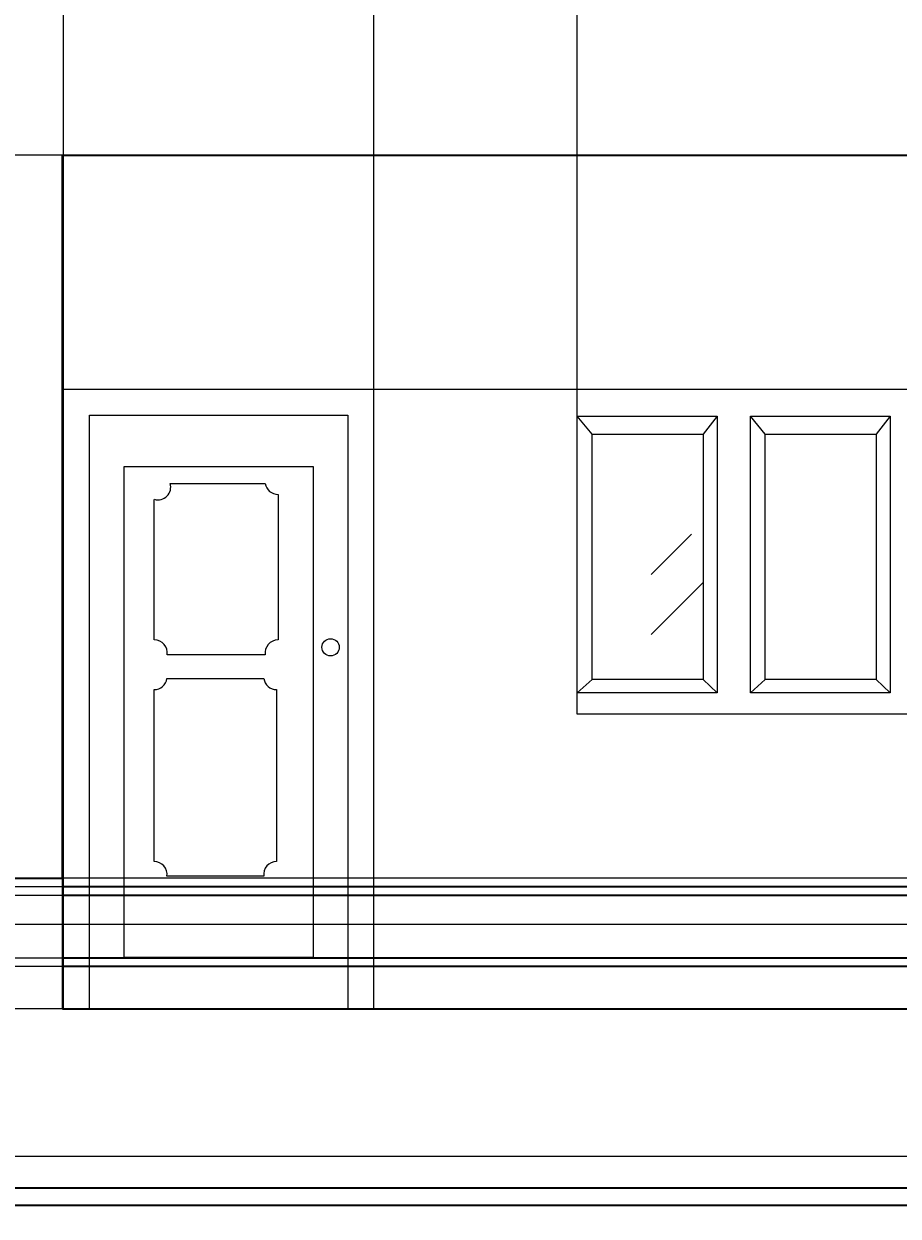
# Model space of a CAD drawing. Units: inches. Extents: x 93 to 565, y 123 to 656.
# Tile 9 of 18: x 291 to 393, y 324 to 463. Entities that reach past the tile are written whole.
import ezdxf

# ---------------------------------------------------------------- set-up
doc = ezdxf.new("R2010")
doc.units = ezdxf.units.IN
doc.header["$MEASUREMENT"] = 0
for name, color, linetype, lineweight in [('A-ANNO-DIMS', 2, 'Continuous', 18), ('A-DOOR', 3, 'Continuous', 25), ('A-ELEV', 7, 'Continuous', 35), ('A-GLAZ', 4, 'Continuous', 25)]:
    doc.layers.add(name, color=color, linetype=linetype, lineweight=lineweight)
doc.styles.get("Standard").update_dxf_attribs({"font": 'arial.ttf'})
doc.dimstyles.get("Standard").update_dxf_attribs({"dimtxt": 0.18, "dimasz": 0.18, "dimexe": 0.18, "dimexo": 0.0625, "dimgap": 0.09, "dimtad": 0, "dimtih": 1, "dimtoh": 1, "dimdec": 4, "dimzin": 0, "dimdsep": 46, "dimtxsty": 'Standard', "dimcen": 0.09, "dimadec": 0, "dimazin": 0, "dimtfac": 1, "dimtdec": 4, "dimtofl": 0, "dimtmove": 0, "dimatfit": 3, "dimfxl": 1, "dimtolj": 1, "dimtzin": 0, "dimarcsym": 0})

# ---------------------------------------------------------------- blocks, each defined once
blk = doc.blocks.new('*U10')
blk.add_lwpolyline([(3.12, 0.01), (0.12, 0.01), (0.12, 72.01), (36.12, 72.01), (36.12, 0.01), (33.12, 0.01)])
for points in [[(33.12, 68.99), (33.12, 0.01), (3.12, 0.01), (3.12, 68.99)], [(29.12, 6.01), (29.12, 62.99), (7.12, 62.99), (7.12, 6.01)]]:
    blk.add_lwpolyline(points, close=True)
blk.add_circle((31.12, 42.01), 1)
blk = doc.blocks.new('DOOR-PANEL-UPPER')
for points in [[(1.85, 19.9), (12.89, 19.9)], [(0, 1.72), (0, 18.05)], [(14.37, 18.62), (14.37, 1.72)], [(12.89, 0), (1.48, 0)]]:
    blk.add_lwpolyline(points)
for centre, start, end in [((0.41, 19.5), 254.1895, 15.8285), ((14.37, 20.12), 188.4141, 270), ((0, 0.22), 351.5859, 90), ((14.37, 0.22), 90, 188.4141)]:
    blk.add_arc(centre, 1.5, start, end)
blk = doc.blocks.new('DOOR-PANEL-LOWER')
for points in [[(1.48, 22.97), (12.73, 22.97)], [(0, 1.72), (0, 21.69)], [(14.21, 21.69), (14.21, 1.72)], [(12.73, 0), (1.48, 0)]]:
    blk.add_lwpolyline(points)
for centre, start, end in [((0, 23.19), 270, 351.5859), ((14.21, 23.19), 188.4141, 270), ((0, 0.22), 351.5859, 90), ((14.21, 0.22), 90, 188.4141)]:
    blk.add_arc(centre, 1.5, start, end)
blk = doc.blocks.new('WIN-CASEMENT-SMALL')
blk.add_lwpolyline([(1.71, 28.48), (0, 30.59), (16.23, 30.59), (14.61, 28.48)])
blk.add_lwpolyline([(1.71, 28.48), (14.61, 28.48), (14.61, 0), (1.71, 0)], close=True)
blk = doc.blocks.new('*D28')
at = {"layer": 'A-ANNO-DIMS', "color": 0, "lineweight": -2, "transparency": 16777216}
for p, q in [((210.54, 519.04), (210.54, 134)), ((295.69, 183.67), (295.69, 134)), ((210.72, 134.18), (252.72, 134.18)), ((295.51, 134.18), (253.51, 134.18))]:
    blk.add_line(p, q, dxfattribs=at)
at = {"layer": 'A-ANNO-DIMS', "color": 0, "transparency": 16777216}
for points in [[(210.72, 134.21), (210.72, 134.15), (210.54, 134.18)], [(295.51, 134.21), (295.51, 134.15), (295.69, 134.18)]]:
    blk.add_solid(points, dxfattribs=at)
at = {"layer": 'Defpoints', "color": 0, "transparency": 16777216}
for p in [(210.54, 519.1), (295.69, 183.73), (295.69, 134.18)]:
    blk.add_point(p, dxfattribs=at)
at = {"layer": 'A-ANNO-DIMS', "color": 0, "transparency": 16777216, "insert": (253.12, 134.18), "char_height": 0.18, "attachment_point": 5}
blk.add_mtext('\\A1;85.14', dxfattribs=at)
blk = doc.blocks.new('*D29')
at = {"layer": 'A-ANNO-DIMS', "color": 0, "lineweight": -2, "transparency": 16777216}
for p, q in [((437.19, 594.34), (437.19, 134)), ((295.69, 183.67), (295.69, 134)), ((295.87, 134.18), (366.05, 134.18)), ((437.01, 134.18), (366.82, 134.18))]:
    blk.add_line(p, q, dxfattribs=at)
at = {"layer": 'A-ANNO-DIMS', "color": 0, "transparency": 16777216}
for points in [[(295.87, 134.21), (295.87, 134.15), (295.69, 134.18)], [(437.01, 134.21), (437.01, 134.15), (437.19, 134.18)]]:
    blk.add_solid(points, dxfattribs=at)
at = {"layer": 'Defpoints', "color": 0, "transparency": 16777216}
for p in [(437.19, 594.4), (295.69, 183.73), (437.19, 134.18)]:
    blk.add_point(p, dxfattribs=at)
at = {"layer": 'A-ANNO-DIMS', "color": 0, "transparency": 16777216, "insert": (366.44, 134.18), "char_height": 0.18, "attachment_point": 5}
blk.add_mtext('\\A1;141.5', dxfattribs=at)
blk = doc.blocks.new('*D31')
at = {"layer": 'A-ANNO-DIMS', "color": 0, "lineweight": -2, "transparency": 16777216}
for p, q in [((417.87, 630.4), (564.81, 630.4)), ((564.63, 630.22), (564.63, 395.25)), ((564.63, 159.91), (564.63, 394.89)), ((119.14, 159.73), (564.81, 159.73))]:
    blk.add_line(p, q, dxfattribs=at)
at = {"layer": 'A-ANNO-DIMS', "color": 0, "transparency": 16777216}
for points in [[(564.6, 630.22), (564.66, 630.22), (564.63, 630.4)], [(564.6, 159.91), (564.66, 159.91), (564.63, 159.73)]]:
    blk.add_solid(points, dxfattribs=at)
at = {"layer": 'Defpoints', "color": 0, "transparency": 16777216}
for p in [(417.81, 630.4), (564.63, 630.4), (119.08, 159.73)]:
    blk.add_point(p, dxfattribs=at)
at = {"layer": 'A-ANNO-DIMS', "color": 0, "transparency": 16777216, "insert": (564.63, 395.07), "char_height": 0.18, "attachment_point": 5}
blk.add_mtext('\\A1;470.7', dxfattribs=at)
blk = doc.blocks.new('*D66')
at = {"layer": 'A-ANNO-DIMS', "color": 0, "lineweight": -2, "transparency": 16777216}
for p, q in [((295.81, 420.63), (295.81, 656.13)), ((295.99, 655.95), (313.59, 655.95)), ((331.63, 655.95), (314.03, 655.95)), ((331.81, 420.63), (331.81, 656.13))]:
    blk.add_line(p, q, dxfattribs=at)
at = {"layer": 'A-ANNO-DIMS', "color": 0, "transparency": 16777216}
for points in [[(295.99, 655.98), (295.99, 655.92), (295.81, 655.95)], [(331.63, 655.98), (331.63, 655.92), (331.81, 655.95)]]:
    blk.add_solid(points, dxfattribs=at)
at = {"layer": 'Defpoints', "color": 0, "transparency": 16777216}
for p in [(331.81, 655.95), (295.81, 420.57), (331.81, 420.57)]:
    blk.add_point(p, dxfattribs=at)
at = {"layer": 'A-ANNO-DIMS', "color": 0, "transparency": 16777216, "insert": (313.81, 655.95), "char_height": 0.18, "attachment_point": 5}
blk.add_mtext('\\A1;36', dxfattribs=at)
blk = doc.blocks.new('*D67')
at = {"layer": 'A-ANNO-DIMS', "color": 0, "lineweight": -2, "transparency": 16777216}
for p, q in [((331.87, 420.57), (564.81, 420.57)), ((564.63, 420.39), (564.63, 384.75)), ((564.63, 348.75), (564.63, 384.39)), ((331.87, 348.57), (564.81, 348.57))]:
    blk.add_line(p, q, dxfattribs=at)
at = {"layer": 'A-ANNO-DIMS', "color": 0, "transparency": 16777216}
for points in [[(564.6, 420.39), (564.66, 420.39), (564.63, 420.57)], [(564.6, 348.75), (564.66, 348.75), (564.63, 348.57)]]:
    blk.add_solid(points, dxfattribs=at)
at = {"layer": 'Defpoints', "color": 0, "transparency": 16777216}
for p in [(331.81, 420.57), (564.63, 420.57), (331.81, 348.57)]:
    blk.add_point(p, dxfattribs=at)
at = {"layer": 'A-ANNO-DIMS', "color": 0, "transparency": 16777216, "insert": (564.63, 384.57), "char_height": 0.18, "attachment_point": 5}
blk.add_mtext('\\A1;72', dxfattribs=at)
blk = doc.blocks.new('*D68')
at = {"layer": 'A-ANNO-DIMS', "color": 0, "lineweight": -2, "transparency": 16777216}
for p, q in [((331.81, 420.63), (331.81, 656.13)), ((331.99, 655.95), (343.24, 655.95)), ((355.28, 655.95), (344.03, 655.95)), ((355.46, 420.63), (355.46, 656.13))]:
    blk.add_line(p, q, dxfattribs=at)
at = {"layer": 'A-ANNO-DIMS', "color": 0, "transparency": 16777216}
for points in [[(331.99, 655.98), (331.99, 655.92), (331.81, 655.95)], [(355.28, 655.98), (355.28, 655.92), (355.46, 655.95)]]:
    blk.add_solid(points, dxfattribs=at)
at = {"layer": 'Defpoints', "color": 0, "transparency": 16777216}
for p in [(355.46, 655.95), (331.81, 420.57), (355.46, 420.57)]:
    blk.add_point(p, dxfattribs=at)
at = {"layer": 'A-ANNO-DIMS', "color": 0, "transparency": 16777216, "insert": (343.64, 655.95), "char_height": 0.18, "attachment_point": 5}
blk.add_mtext('\\A1;23.65', dxfattribs=at)
blk = doc.blocks.new('*D69')
at = {"layer": 'A-ANNO-DIMS', "color": 0, "lineweight": -2, "transparency": 16777216}
for p, q in [((355.46, 420.63), (355.46, 656.13)), ((355.64, 655.95), (391.65, 655.95)), ((428.44, 655.95), (392.43, 655.95)), ((428.62, 420.63), (428.62, 656.13))]:
    blk.add_line(p, q, dxfattribs=at)
at = {"layer": 'A-ANNO-DIMS', "color": 0, "transparency": 16777216}
for points in [[(355.64, 655.98), (355.64, 655.92), (355.46, 655.95)], [(428.44, 655.98), (428.44, 655.92), (428.62, 655.95)]]:
    blk.add_solid(points, dxfattribs=at)
at = {"layer": 'Defpoints', "color": 0, "transparency": 16777216}
for p in [(428.62, 655.95), (355.46, 420.57), (428.62, 420.57)]:
    blk.add_point(p, dxfattribs=at)
at = {"layer": 'A-ANNO-DIMS', "color": 0, "transparency": 16777216, "insert": (392.04, 655.95), "char_height": 0.18, "attachment_point": 5}
blk.add_mtext('\\A1;73.16', dxfattribs=at)
blk = doc.blocks.new('*D72')
at = {"layer": 'A-ANNO-DIMS', "color": 0, "lineweight": -2, "transparency": 16777216}
for p, q in [((295.62, 447.73), (93.35, 447.73)), ((93.53, 447.55), (93.53, 405.91)), ((93.53, 363.91), (93.53, 405.55)), ((286.62, 363.73), (93.35, 363.73))]:
    blk.add_line(p, q, dxfattribs=at)
at = {"layer": 'A-ANNO-DIMS', "color": 0, "transparency": 16777216}
for points in [[(93.5, 447.55), (93.56, 447.55), (93.53, 447.73)], [(93.5, 363.91), (93.56, 363.91), (93.53, 363.73)]]:
    blk.add_solid(points, dxfattribs=at)
at = {"layer": 'Defpoints', "color": 0, "transparency": 16777216}
for p in [(295.69, 447.73), (93.53, 363.73), (286.69, 363.73)]:
    blk.add_point(p, dxfattribs=at)
at = {"layer": 'A-ANNO-DIMS', "color": 0, "transparency": 16777216, "insert": (93.53, 405.73), "char_height": 0.18, "attachment_point": 5}
blk.add_mtext('\\A1;84', dxfattribs=at)
blk = doc.blocks.new('*D107')
at = {"layer": 'A-ANNO-DIMS', "color": 0, "lineweight": -2, "transparency": 16777216}
for p, q in [((210.54, 519.04), (210.54, 134)), ((295.69, 183.67), (295.69, 134)), ((210.72, 134.18), (252.65, 134.18)), ((295.51, 134.18), (253.58, 134.18))]:
    blk.add_line(p, q, dxfattribs=at)
at = {"layer": 'A-ANNO-DIMS', "color": 0, "transparency": 16777216}
for points in [[(210.72, 134.21), (210.72, 134.15), (210.54, 134.18)], [(295.51, 134.21), (295.51, 134.15), (295.69, 134.18)]]:
    blk.add_solid(points, dxfattribs=at)
at = {"layer": 'Defpoints', "color": 0, "transparency": 16777216}
for p in [(210.54, 519.1), (295.69, 183.73), (295.69, 134.18)]:
    blk.add_point(p, dxfattribs=at)
at = {"layer": 'A-ANNO-DIMS', "color": 0, "transparency": 16777216, "insert": (253.12, 134.18), "char_height": 0.18, "attachment_point": 5}
blk.add_mtext('\\A1;85.143', dxfattribs=at)
blk = doc.blocks.new('*D108')
at = {"layer": 'A-ANNO-DIMS', "color": 0, "lineweight": -2, "transparency": 16777216}
for p, q in [((437.19, 594.34), (437.19, 134)), ((295.69, 183.67), (295.69, 134)), ((295.87, 134.18), (365.93, 134.18)), ((437.01, 134.18), (366.95, 134.18))]:
    blk.add_line(p, q, dxfattribs=at)
at = {"layer": 'A-ANNO-DIMS', "color": 0, "transparency": 16777216}
for points in [[(295.87, 134.21), (295.87, 134.15), (295.69, 134.18)], [(437.01, 134.21), (437.01, 134.15), (437.19, 134.18)]]:
    blk.add_solid(points, dxfattribs=at)
at = {"layer": 'Defpoints', "color": 0, "transparency": 16777216}
for p in [(437.19, 594.4), (295.69, 183.73), (437.19, 134.18)]:
    blk.add_point(p, dxfattribs=at)
at = {"layer": 'A-ANNO-DIMS', "color": 0, "transparency": 16777216, "insert": (366.44, 134.18), "char_height": 0.18, "attachment_point": 5}
blk.add_mtext('\\A1;141.501', dxfattribs=at)
blk = doc.blocks.new('*D110')
at = {"layer": 'A-ANNO-DIMS', "color": 0, "lineweight": -2, "transparency": 16777216}
for p, q in [((417.87, 630.4), (564.81, 630.4)), ((564.63, 630.22), (564.63, 395.25)), ((564.63, 159.91), (564.63, 394.89)), ((119.14, 159.73), (564.81, 159.73))]:
    blk.add_line(p, q, dxfattribs=at)
at = {"layer": 'A-ANNO-DIMS', "color": 0, "transparency": 16777216}
for points in [[(564.6, 630.22), (564.66, 630.22), (564.63, 630.4)], [(564.6, 159.91), (564.66, 159.91), (564.63, 159.73)]]:
    blk.add_solid(points, dxfattribs=at)
at = {"layer": 'Defpoints', "color": 0, "transparency": 16777216}
for p in [(417.81, 630.4), (564.63, 630.4), (119.08, 159.73)]:
    blk.add_point(p, dxfattribs=at)
at = {"layer": 'A-ANNO-DIMS', "color": 0, "transparency": 16777216, "insert": (564.63, 395.07), "char_height": 0.18, "attachment_point": 5}
blk.add_mtext('\\A1;470.673', dxfattribs=at)
blk = doc.blocks.new('*D145')
at = {"layer": 'A-ANNO-DIMS', "color": 0, "lineweight": -2, "transparency": 16777216}
for p, q in [((295.81, 420.63), (295.81, 656.13)), ((295.99, 655.95), (313.35, 655.95)), ((331.63, 655.95), (314.27, 655.95)), ((331.81, 420.63), (331.81, 656.13))]:
    blk.add_line(p, q, dxfattribs=at)
at = {"layer": 'A-ANNO-DIMS', "color": 0, "transparency": 16777216}
for points in [[(295.99, 655.98), (295.99, 655.92), (295.81, 655.95)], [(331.63, 655.98), (331.63, 655.92), (331.81, 655.95)]]:
    blk.add_solid(points, dxfattribs=at)
at = {"layer": 'Defpoints', "color": 0, "transparency": 16777216}
for p in [(331.81, 655.95), (295.81, 420.57), (331.81, 420.57)]:
    blk.add_point(p, dxfattribs=at)
at = {"layer": 'A-ANNO-DIMS', "color": 0, "transparency": 16777216, "insert": (313.81, 655.95), "char_height": 0.18, "attachment_point": 5}
blk.add_mtext('\\A1;36.000', dxfattribs=at)
blk = doc.blocks.new('*D146')
at = {"layer": 'A-ANNO-DIMS', "color": 0, "lineweight": -2, "transparency": 16777216}
for p, q in [((331.87, 420.57), (564.81, 420.57)), ((564.63, 420.39), (564.63, 384.75)), ((564.63, 348.75), (564.63, 384.39)), ((331.87, 348.57), (564.81, 348.57))]:
    blk.add_line(p, q, dxfattribs=at)
at = {"layer": 'A-ANNO-DIMS', "color": 0, "transparency": 16777216}
for points in [[(564.6, 420.39), (564.66, 420.39), (564.63, 420.57)], [(564.6, 348.75), (564.66, 348.75), (564.63, 348.57)]]:
    blk.add_solid(points, dxfattribs=at)
at = {"layer": 'Defpoints', "color": 0, "transparency": 16777216}
for p in [(331.81, 420.57), (564.63, 420.57), (331.81, 348.57)]:
    blk.add_point(p, dxfattribs=at)
at = {"layer": 'A-ANNO-DIMS', "color": 0, "transparency": 16777216, "insert": (564.63, 384.57), "char_height": 0.18, "attachment_point": 5}
blk.add_mtext('\\A1;72.000', dxfattribs=at)
blk = doc.blocks.new('*D147')
at = {"layer": 'A-ANNO-DIMS', "color": 0, "lineweight": -2, "transparency": 16777216}
for p, q in [((331.81, 420.63), (331.81, 656.13)), ((331.99, 655.95), (343.17, 655.95)), ((355.28, 655.95), (344.1, 655.95)), ((355.46, 420.63), (355.46, 656.13))]:
    blk.add_line(p, q, dxfattribs=at)
at = {"layer": 'A-ANNO-DIMS', "color": 0, "transparency": 16777216}
for points in [[(331.99, 655.98), (331.99, 655.92), (331.81, 655.95)], [(355.28, 655.98), (355.28, 655.92), (355.46, 655.95)]]:
    blk.add_solid(points, dxfattribs=at)
at = {"layer": 'Defpoints', "color": 0, "transparency": 16777216}
for p in [(355.46, 655.95), (331.81, 420.57), (355.46, 420.57)]:
    blk.add_point(p, dxfattribs=at)
at = {"layer": 'A-ANNO-DIMS', "color": 0, "transparency": 16777216, "insert": (343.64, 655.95), "char_height": 0.18, "attachment_point": 5}
blk.add_mtext('\\A1;23.649', dxfattribs=at)
blk = doc.blocks.new('*D148')
at = {"layer": 'A-ANNO-DIMS', "color": 0, "lineweight": -2, "transparency": 16777216}
for p, q in [((355.46, 420.63), (355.46, 656.13)), ((355.64, 655.95), (391.58, 655.95)), ((428.44, 655.95), (392.5, 655.95)), ((428.62, 420.63), (428.62, 656.13))]:
    blk.add_line(p, q, dxfattribs=at)
at = {"layer": 'A-ANNO-DIMS', "color": 0, "transparency": 16777216}
for points in [[(355.64, 655.98), (355.64, 655.92), (355.46, 655.95)], [(428.44, 655.98), (428.44, 655.92), (428.62, 655.95)]]:
    blk.add_solid(points, dxfattribs=at)
at = {"layer": 'Defpoints', "color": 0, "transparency": 16777216}
for p in [(428.62, 655.95), (355.46, 420.57), (428.62, 420.57)]:
    blk.add_point(p, dxfattribs=at)
at = {"layer": 'A-ANNO-DIMS', "color": 0, "transparency": 16777216, "insert": (392.04, 655.95), "char_height": 0.18, "attachment_point": 5}
blk.add_mtext('\\A1;73.156', dxfattribs=at)
blk = doc.blocks.new('*D151')
at = {"layer": 'A-ANNO-DIMS', "color": 0, "lineweight": -2, "transparency": 16777216}
for p, q in [((295.62, 447.73), (93.35, 447.73)), ((93.53, 447.55), (93.53, 405.91)), ((93.53, 363.91), (93.53, 405.55)), ((286.62, 363.73), (93.35, 363.73))]:
    blk.add_line(p, q, dxfattribs=at)
at = {"layer": 'A-ANNO-DIMS', "color": 0, "transparency": 16777216}
for points in [[(93.5, 447.55), (93.56, 447.55), (93.53, 447.73)], [(93.5, 363.91), (93.56, 363.91), (93.53, 363.73)]]:
    blk.add_solid(points, dxfattribs=at)
at = {"layer": 'Defpoints', "color": 0, "transparency": 16777216}
for p in [(295.69, 447.73), (93.53, 363.73), (286.69, 363.73)]:
    blk.add_point(p, dxfattribs=at)
at = {"layer": 'A-ANNO-DIMS', "color": 0, "transparency": 16777216, "insert": (93.53, 405.73), "char_height": 0.18, "attachment_point": 5}
blk.add_mtext('\\A1;84.000', dxfattribs=at)
blk = doc.blocks.new('*D190')
at = {"layer": 'A-ANNO-DIMS', "color": 0, "lineweight": -2, "transparency": 16777216}
for p, q in [((514.58, 348.55), (93.35, 348.55)), ((93.53, 348.37), (93.53, 338.33)), ((93.53, 327.91), (93.53, 337.96)), ((539.02, 327.73), (93.35, 327.73))]:
    blk.add_line(p, q, dxfattribs=at)
at = {"layer": 'A-ANNO-DIMS', "color": 0, "transparency": 16777216}
for points in [[(93.5, 348.37), (93.56, 348.37), (93.53, 348.55)], [(93.5, 327.91), (93.56, 327.91), (93.53, 327.73)]]:
    blk.add_solid(points, dxfattribs=at)
at = {"layer": 'Defpoints', "color": 0, "transparency": 16777216}
for p in [(93.53, 348.55), (514.64, 348.55), (539.08, 327.73)]:
    blk.add_point(p, dxfattribs=at)
at = {"layer": 'A-ANNO-DIMS', "color": 0, "transparency": 16777216, "insert": (93.53, 338.14), "char_height": 0.18, "attachment_point": 5}
blk.add_mtext('\\A1;20.822', dxfattribs=at)
blk = doc.blocks.new('*D191')
at = {"layer": 'A-ANNO-DIMS', "color": 0, "lineweight": -2, "transparency": 16777216}
for p, q in [((514.58, 353.47), (93.35, 353.47)), ((93.53, 353.29), (93.53, 351.2)), ((93.53, 348.73), (93.53, 350.83)), ((514.58, 348.55), (93.35, 348.55))]:
    blk.add_line(p, q, dxfattribs=at)
at = {"layer": 'A-ANNO-DIMS', "color": 0, "transparency": 16777216}
for points in [[(93.5, 353.29), (93.56, 353.29), (93.53, 353.47)], [(93.5, 348.73), (93.56, 348.73), (93.53, 348.55)]]:
    blk.add_solid(points, dxfattribs=at)
at = {"layer": 'Defpoints', "color": 0, "transparency": 16777216}
for p in [(93.53, 353.47), (514.64, 353.47), (514.64, 348.55)]:
    blk.add_point(p, dxfattribs=at)
at = {"layer": 'A-ANNO-DIMS', "color": 0, "transparency": 16777216, "insert": (93.53, 351.01), "char_height": 0.18, "attachment_point": 5}
blk.add_mtext('\\A1;4.918', dxfattribs=at)
blk = doc.blocks.new('*D192')
at = {"layer": 'A-ANNO-DIMS', "color": 0, "lineweight": -2, "transparency": 16777216}
for p, q in [((514.58, 354.47), (93.35, 354.47)), ((514.58, 353.47), (93.35, 353.47)), ((93.53, 354.29), (93.53, 354.15)), ((93.53, 353.65), (93.53, 353.79))]:
    blk.add_line(p, q, dxfattribs=at)
at = {"layer": 'A-ANNO-DIMS', "color": 0, "transparency": 16777216}
for points in [[(93.5, 354.29), (93.56, 354.29), (93.53, 354.47)], [(93.5, 353.65), (93.56, 353.65), (93.53, 353.47)]]:
    blk.add_solid(points, dxfattribs=at)
at = {"layer": 'Defpoints', "color": 0, "transparency": 16777216}
for p in [(93.53, 354.47), (514.64, 354.47), (514.64, 353.47)]:
    blk.add_point(p, dxfattribs=at)
at = {"layer": 'A-ANNO-DIMS', "color": 0, "transparency": 16777216, "insert": (93.53, 353.97), "char_height": 0.18, "attachment_point": 5}
blk.add_mtext('\\A1;1.000', dxfattribs=at)
blk = doc.blocks.new('*D193')
at = {"layer": 'A-ANNO-DIMS', "color": 0, "lineweight": -2, "transparency": 16777216}
for p, q in [((514.58, 358.37), (93.35, 358.37)), ((93.53, 358.19), (93.53, 356.61)), ((93.53, 354.65), (93.53, 356.24)), ((514.58, 354.47), (93.35, 354.47))]:
    blk.add_line(p, q, dxfattribs=at)
at = {"layer": 'A-ANNO-DIMS', "color": 0, "transparency": 16777216}
for points in [[(93.5, 358.19), (93.56, 358.19), (93.53, 358.37)], [(93.5, 354.65), (93.56, 354.65), (93.53, 354.47)]]:
    blk.add_solid(points, dxfattribs=at)
at = {"layer": 'Defpoints', "color": 0, "transparency": 16777216}
for p in [(93.53, 358.37), (514.64, 358.37), (514.64, 354.47)]:
    blk.add_point(p, dxfattribs=at)
at = {"layer": 'A-ANNO-DIMS', "color": 0, "transparency": 16777216, "insert": (93.53, 356.42), "char_height": 0.18, "attachment_point": 5}
blk.add_mtext('\\A1;3.901', dxfattribs=at)
blk = doc.blocks.new('*D194')
at = {"layer": 'A-ANNO-DIMS', "color": 0, "lineweight": -2, "transparency": 16777216}
for p, q in [((524.92, 361.75), (93.35, 361.75)), ((93.53, 361.57), (93.53, 360.24)), ((93.53, 358.55), (93.53, 359.88)), ((514.58, 358.37), (93.35, 358.37))]:
    blk.add_line(p, q, dxfattribs=at)
at = {"layer": 'A-ANNO-DIMS', "color": 0, "transparency": 16777216}
for points in [[(93.5, 361.57), (93.56, 361.57), (93.53, 361.75)], [(93.5, 358.55), (93.56, 358.55), (93.53, 358.37)]]:
    blk.add_solid(points, dxfattribs=at)
at = {"layer": 'Defpoints', "color": 0, "transparency": 16777216}
for p in [(93.53, 361.75), (524.99, 361.75), (514.64, 358.37)]:
    blk.add_point(p, dxfattribs=at)
at = {"layer": 'A-ANNO-DIMS', "color": 0, "transparency": 16777216, "insert": (93.53, 360.06), "char_height": 0.18, "attachment_point": 5}
blk.add_mtext('\\A1;3.374', dxfattribs=at)
blk = doc.blocks.new('*D195')
at = {"layer": 'A-ANNO-DIMS', "color": 0, "lineweight": -2, "transparency": 16777216}
for p, q in [((524.92, 362.75), (93.35, 362.75)), ((524.92, 361.75), (93.35, 361.75)), ((93.53, 362.57), (93.53, 362.43)), ((93.53, 361.93), (93.53, 362.07))]:
    blk.add_line(p, q, dxfattribs=at)
at = {"layer": 'A-ANNO-DIMS', "color": 0, "transparency": 16777216}
for points in [[(93.5, 362.57), (93.56, 362.57), (93.53, 362.75)], [(93.5, 361.93), (93.56, 361.93), (93.53, 361.75)]]:
    blk.add_solid(points, dxfattribs=at)
at = {"layer": 'Defpoints', "color": 0, "transparency": 16777216}
for p in [(93.53, 362.75), (524.99, 362.75), (524.99, 361.75)]:
    blk.add_point(p, dxfattribs=at)
at = {"layer": 'A-ANNO-DIMS', "color": 0, "transparency": 16777216, "insert": (93.53, 362.25), "char_height": 0.18, "attachment_point": 5}
blk.add_mtext('\\A1;1.000', dxfattribs=at)
blk = doc.blocks.new('*D196')
at = {"layer": 'A-ANNO-DIMS', "color": 0, "lineweight": -2, "transparency": 16777216}
for p, q in [((524.92, 363.73), (93.35, 363.73)), ((93.53, 363.55), (93.53, 363.42)), ((93.53, 362.93), (93.53, 363.06)), ((524.92, 362.75), (93.35, 362.75))]:
    blk.add_line(p, q, dxfattribs=at)
at = {"layer": 'A-ANNO-DIMS', "color": 0, "transparency": 16777216}
for points in [[(93.5, 363.55), (93.56, 363.55), (93.53, 363.73)], [(93.5, 362.93), (93.56, 362.93), (93.53, 362.75)]]:
    blk.add_solid(points, dxfattribs=at)
at = {"layer": 'Defpoints', "color": 0, "transparency": 16777216}
for p in [(93.53, 363.73), (524.99, 363.73), (524.99, 362.75)]:
    blk.add_point(p, dxfattribs=at)
at = {"layer": 'A-ANNO-DIMS', "color": 0, "transparency": 16777216, "insert": (93.53, 363.24), "char_height": 0.18, "attachment_point": 5}
blk.add_mtext('\\A1;0.985', dxfattribs=at)
blk = doc.blocks.new('*D198')
at = {"layer": 'A-ANNO-DIMS', "color": 0, "lineweight": -2, "transparency": 16777216}
for p, q in [((515.95, 331.43), (93.35, 331.43)), ((93.53, 331.25), (93.53, 329.76)), ((93.53, 327.91), (93.53, 329.4)), ((539.02, 327.73), (93.35, 327.73))]:
    blk.add_line(p, q, dxfattribs=at)
at = {"layer": 'A-ANNO-DIMS', "color": 0, "transparency": 16777216}
for points in [[(93.5, 331.25), (93.56, 331.25), (93.53, 331.43)], [(93.5, 327.91), (93.56, 327.91), (93.53, 327.73)]]:
    blk.add_solid(points, dxfattribs=at)
at = {"layer": 'Defpoints', "color": 0, "transparency": 16777216}
for p in [(93.53, 331.43), (516.01, 331.43), (539.08, 327.73)]:
    blk.add_point(p, dxfattribs=at)
at = {"layer": 'A-ANNO-DIMS', "color": 0, "transparency": 16777216, "insert": (93.53, 329.58), "char_height": 0.18, "attachment_point": 5}
blk.add_mtext('\\A1;3.701', dxfattribs=at)

msp = doc.modelspace()

# ---------------------------------------------------------------- hatches: boundary and pattern name
at = {"layer": 'A-GLAZ'}
h = msp.add_hatch(dxfattribs=at)
h.set_pattern_fill('GOST_GLASS', color=256, scale=3.3)
h.set_pattern_definition([(45, (0, 0), (28.0014, 0), [16.5, -23.1]), (45, (7, 0), (28.0014, 0), [6.6, -33]), (45, (0, 7), (28.0014, 0), [6.6, -33])])
h.paths.add_polyline_path([(332.6288, 267.5414), (312.4161, 267.5414), (312.4161, 222.941), (332.6288, 222.941)])
h.paths.add_polyline_path([(370.0743, 415.3107), (357.167, 415.3107), (357.167, 386.8299), (370.0743, 386.8299)])
h.paths.add_polyline_path([(390.168, 415.3107), (377.2607, 415.3107), (377.2607, 386.8299), (390.168, 386.8299)])
h.paths.add_polyline_path([(408.2592, 415.3107), (395.3518, 415.3107), (395.3518, 386.8299), (408.2592, 386.8299)])
h.paths.add_polyline_path([(427.0129, 415.3107), (414.1056, 415.3107), (414.1056, 386.8299), (427.0129, 386.8299)])

# ---------------------------------------------------------------- linework, layer by layer
at = {"layer": 'A-ELEV'}
for p, q in [((295.6874, 363.7323), (295.6874, 447.7323)), ((295.6874, 447.7323), (437.1885, 447.7323)), ((286.6874, 363.7323), (295.6874, 363.7323)), ((295.6874, 363.7323), (295.6874, 348.5546)), ((524.9864, 362.7477), (295.6874, 362.7477)), ((524.9864, 361.7477), (295.6874, 361.7477)), ((514.6424, 354.4729), (295.6874, 354.4729)), ((514.6424, 353.4729), (295.6874, 353.4729)), ((295.6874, 348.5546), (514.6424, 348.5546)), ((295.6874, 327.7323), (286.6874, 327.7323)), ((539.0794, 327.7323), (295.6874, 327.7323)), ((295.6874, 325.7323), (286.6874, 325.7323)), ((539.0794, 325.7323), (295.6874, 325.7323))]:
    msp.add_line(p, q, dxfattribs=at)
at = {"layer": 'A-GLAZ'}
for p, q in [((371.6921, 385.2642), (355.4603, 385.2642)), ((391.7858, 385.2642), (375.5539, 385.2642))]:
    msp.add_line(p, q, dxfattribs=at)
msp.add_lwpolyline([(355.4603, 420.5674), (428.6158, 420.5674), (428.6158, 382.7996), (355.4603, 382.7996)], close=True, dxfattribs=at)
for points in [[(357.167, 386.8299), (355.4603, 385.2642), (355.4603, 417.4228)], [(371.6921, 417.4228), (371.6921, 385.2642), (370.0743, 386.8299)], [(377.2607, 386.8299), (375.5539, 385.2642), (375.5539, 417.4228)], [(391.7858, 417.4228), (391.7858, 385.2642), (390.168, 386.8299)]]:
    msp.add_lwpolyline(points, dxfattribs=at)

# ---------------------------------------------------------------- block references
at = {"layer": 'A-DOOR'}
for name, p in [('*U10', (295.6874, 348.5546)), ('DOOR-PANEL-UPPER', (306.3374, 389.6978)), ('DOOR-PANEL-LOWER', (306.3252, 363.9605))]:
    msp.add_blockref(name, p, dxfattribs=at)
at = {"layer": 'A-GLAZ'}
for p in [(355.46, 386.83), (375.5537, 386.83)]:
    msp.add_blockref('WIN-CASEMENT-SMALL', p, dxfattribs=at)

# ---------------------------------------------------------------- dimensions: what is measured, and where the dimension line sits
at = {"layer": 'A-ANNO-DIMS'}
for base, p1, p2, override, picture, middle in [((331.8112, 655.9548), (295.8112, 420.5674), (331.8112, 420.5674), {"dimdec": 0, "dimlfac": 1, "dimrnd": 0, "dimzin": 0, "dimdsep": 46, "dimlunit": 2}, '*D66', (313.8112, 655.9548)), ((331.8112, 655.9548), (295.8112, 420.5674), (331.8112, 420.5674), {"dimdec": 3, "dimlfac": 1, "dimrnd": 0, "dimzin": 0, "dimdsep": 46, "dimlunit": 2}, '*D145', (313.8112, 655.9548)), ((355.4603, 655.9548), (331.8112, 420.5674), (355.4603, 420.5674), {"dimdec": 2, "dimlfac": 1, "dimrnd": 0, "dimzin": 0, "dimdsep": 46, "dimlunit": 2}, '*D68', (343.6357, 655.9548)), ((355.4603, 655.9548), (331.8112, 420.5674), (355.4603, 420.5674), {"dimdec": 3, "dimlfac": 1, "dimrnd": 0, "dimzin": 0, "dimdsep": 46, "dimlunit": 2}, '*D147', (343.6357, 655.9548)), ((428.6158, 655.9548), (355.4603, 420.5674), (428.6158, 420.5674), {"dimdec": 2, "dimlfac": 1, "dimrnd": 0, "dimzin": 0, "dimdsep": 46, "dimlunit": 2}, '*D69', (392.038, 655.9548)), ((428.615792, 655.954775), (355.460288, 420.567351), (428.615792, 420.567351), {"dimdec": 3, "dimlfac": 1, "dimrnd": 0, "dimzin": 0, "dimdsep": 46, "dimlunit": 2}, '*D148', (392.03804, 655.954775)), ((437.1885, 134.1823), (295.6874, 183.7323), (437.1885, 594.4048), {"dimdec": 1, "dimlfac": 1, "dimrnd": 0, "dimzin": 0, "dimdsep": 46, "dimlunit": 2}, '*D29', (366.438, 134.1823)), ((437.1885, 134.1823), (295.6874, 183.7323), (437.1885, 594.4048), {"dimdec": 3, "dimlfac": 1, "dimrnd": 0, "dimzin": 0, "dimdsep": 46, "dimlunit": 2}, '*D108', (366.438, 134.1823)), ((295.6874, 134.1823), (210.5443, 519.0999), (295.6874, 183.7323), {"dimdec": 2, "dimlfac": 1, "dimrnd": 0, "dimzin": 0, "dimdsep": 46, "dimlunit": 2}, '*D28', (253.1158, 134.1823)), ((295.6874, 134.1823), (210.5443, 519.0999), (295.6874, 183.7323), {"dimdec": 3, "dimlfac": 1, "dimrnd": 0, "dimzin": 0, "dimdsep": 46, "dimlunit": 2}, '*D107', (253.1158, 134.1823))]:
    dim = msp.add_linear_dim(base=base, p1=p1, p2=p2, dimstyle='Standard', override=override, dxfattribs=at)
    dim.commit()
    dim.dimension.update_dxf_attribs({"geometry": picture, "text_midpoint": middle})
for base, p1, p2, override, picture, middle in [((564.6294, 630.4048), (119.0794, 159.7323), (417.8097, 630.4048), {"dimdec": 1, "dimlfac": 1, "dimrnd": 0, "dimzin": 0, "dimdsep": 46, "dimlunit": 2}, '*D31', (564.6294, 395.0685)), ((564.62936, 630.40478), (119.07936, 159.73225), (417.80971, 630.40477), {"dimdec": 3, "dimlfac": 1, "dimrnd": 0, "dimzin": 0, "dimdsep": 46, "dimlunit": 2}, '*D110', (564.62936, 395.06851)), ((93.5294, 363.7323), (295.6874, 447.7323), (286.6874, 363.7323), {"dimdec": 3, "dimlfac": 1, "dimrnd": 0, "dimzin": 0, "dimdsep": 46, "dimlunit": 2}, '*D151', (93.5294, 405.7323)), ((93.5294, 363.7323), (295.6874, 447.7323), (286.6874, 363.7323), {"dimdec": 0, "dimlfac": 1, "dimrnd": 0, "dimzin": 0, "dimdsep": 46, "dimlunit": 2}, '*D72', (93.5294, 405.7323)), ((564.6294, 420.5674), (331.8112, 348.5674), (331.8112, 420.5674), {"dimdec": 0, "dimlfac": 1, "dimrnd": 0, "dimzin": 0, "dimdsep": 46, "dimlunit": 2}, '*D67', (564.6294, 384.5674)), ((564.6294, 420.5674), (331.8112, 348.5674), (331.8112, 420.5674), {"dimdec": 3, "dimlfac": 1, "dimrnd": 0, "dimzin": 0, "dimdsep": 46, "dimlunit": 2}, '*D146', (564.6294, 384.5674)), ((93.5294, 363.7323), (524.9864, 362.7477), (524.9864, 363.7323), {"dimdec": 3, "dimlfac": 1, "dimrnd": 0, "dimzin": 0, "dimdsep": 46, "dimlunit": 2}, '*D196', (93.5294, 363.24)), ((93.5294, 362.7477), (524.9864, 361.7477), (524.9864, 362.7477), {"dimdec": 3, "dimlfac": 1, "dimrnd": 0, "dimzin": 0, "dimdsep": 46, "dimlunit": 2}, '*D195', (93.5294, 362.2477)), ((93.5294, 361.7477), (514.6424, 358.3735), (524.9864, 361.7477), {"dimdec": 3, "dimlfac": 1, "dimrnd": 0, "dimzin": 0, "dimdsep": 46, "dimlunit": 2}, '*D194', (93.5294, 360.0606)), ((93.5294, 358.3735), (514.6424, 354.4729), (514.6424, 358.3735), {"dimdec": 3, "dimlfac": 1, "dimrnd": 0, "dimzin": 0, "dimdsep": 46, "dimlunit": 2}, '*D193', (93.5294, 356.4232)), ((93.5294, 354.4729), (514.6424, 353.4729), (514.6424, 354.4729), {"dimdec": 3, "dimlfac": 1, "dimrnd": 0, "dimzin": 0, "dimdsep": 46, "dimlunit": 2}, '*D192', (93.5294, 353.9729)), ((93.5294, 353.4729), (514.6424, 348.5546), (514.6424, 353.4729), {"dimdec": 3, "dimlfac": 1, "dimrnd": 0, "dimzin": 0, "dimdsep": 46, "dimlunit": 2}, '*D191', (93.5294, 351.0137)), ((93.5294, 348.5546), (539.0794, 327.7323), (514.6424, 348.5546), {"dimdec": 3, "dimlfac": 1, "dimrnd": 0, "dimzin": 0, "dimdsep": 46, "dimlunit": 2}, '*D190', (93.5294, 338.1434)), ((93.5294, 331.4335), (539.0794, 327.7323), (516.0099, 331.4335), {"dimdec": 3, "dimlfac": 1, "dimrnd": 0, "dimzin": 0, "dimdsep": 46, "dimlunit": 2}, '*D198', (93.5294, 329.5829))]:
    dim = msp.add_linear_dim(base=base, p1=p1, p2=p2, angle=90, dimstyle='Standard', override=override, dxfattribs=at)
    dim.commit()
    dim.dimension.update_dxf_attribs({"geometry": picture, "text_midpoint": middle})

doc.saveas('drawing.dxf')
